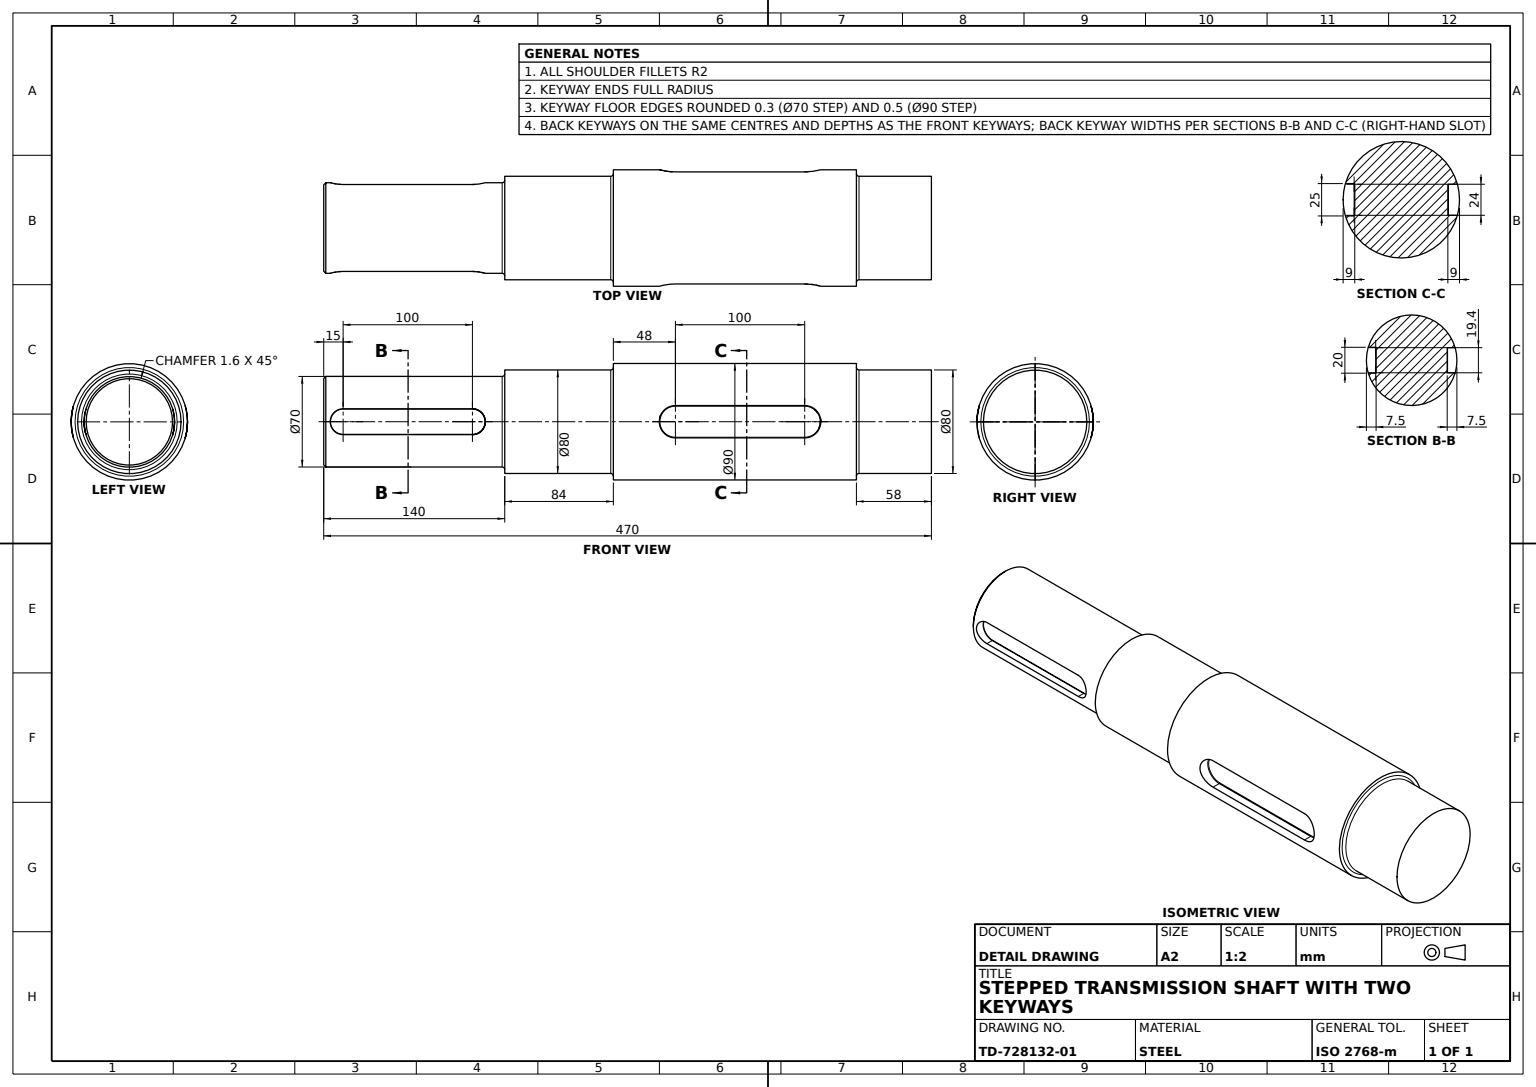
SolidWorks part; units mm, degrees
material "Plain Carbon Steel"
ref_plane "Front Plane" through (0, 0, 0) normal (0, 0, 1) x (1, 0, 0)
ref_plane "Top Plane" through (0, 0, 0) normal (0, 1, 0) x (1, 0, 0)
ref_plane "Right Plane" through (0, 0, 0) normal (1, 0, 0) x (0, 0, -1)
sketch "Shaft Profile Sketch" plane through (0, 0, 0) normal (0, 0, 1) x (1, 0, 0)
  line L0 (0, 0) -> (470, 0) construction
  line L1 (0, 0) -> (0, 35)
  line L2 (0, 35) -> (140, 35)
  line L3 (140, 35) -> (140, 40)
  line L4 (140, 40) -> (224, 40)
  line L5 (224, 40) -> (224, 45)
  line L6 (224, 45) -> (412, 45)
  line L7 (412, 45) -> (412, 40)
  line L8 (412, 40) -> (470, 40)
  line L9 (470, 40) -> (470, 0)
  line L10 (0, 0) -> (470, 0)
  dimension "D1" = 40
  dimension "D2" = 58
  dimension "D3" = 45
  dimension "D4" = 188
  dimension "D5" = 84
  dimension "D6" = 40
  dimension "D7" = 140
  dimension "D8" = 35
revolve "Stepped Shaft Body" add sketch "Shaft Profile Sketch" angle 360 about L0
chamfer "End Chamfer 1.6x45deg" distance 1.6 angle 45 1 edges at (0, 0, 35)
ref_plane "Keyway A Plane" through (0, 0, 35) normal (0, 0, 1) x (1, 0, 0)
sketch "Keyway A Sketch" plane through (0, 0, 35) normal (0, 0, 1) x (1, 0, 0)
  line L0 (15, 0) -> (115, 0) construction
  line L1 (15, 10) -> (115, 10)
  line L2 (15, -10) -> (115, -10)
  line L3 (0, 33.4) -> (0, -33.4) construction
  arc A0 (15, 10) -> (15, -10) centre (15, 0) ccw
  arc A1 (115, -10) -> (115, 10) centre (115, 0) ccw
  point P3 (65, 0)
  dimension "D2" = 10
  dimension "D1" = 100
  dimension "D3" = 15
extrude "Keyway A Cut 7.5 Deep" cut sketch "Keyway A Sketch" against normal blind 7.5
fillet "Keyway A Edge Fillet R0.3" radius 0.3 4 edges at (125, 0, 27.5) (65, -10, 27.5) (5, 0, 27.5) (65, 10, 27.5)
ref_plane "Keyway B Plane" through (0, 0, 45) normal (0, 0, 1) x (1, 0, 0)
sketch "Keyway B Sketch" plane through (0, 0, 45) normal (0, 0, 1) x (1, 0, 0)
  line L0 (272, 0) -> (372, 0) construction
  line L1 (272, 12.5) -> (372, 12.5)
  line L2 (272, -12.5) -> (372, -12.5)
  line L3 (412, -40) -> (412, 40) construction
  arc A0 (272, 12.5) -> (272, -12.5) centre (272, 0) ccw
  arc A1 (372, -12.5) -> (372, 12.5) centre (372, 0) ccw
  point P3 (322, 0)
  dimension "D2" = 12.5
  dimension "D1" = 100
  dimension "D3" = 40
extrude "Keyway B Cut 9 Deep" cut sketch "Keyway B Sketch" against normal blind 9
fillet "Keyway B Edge Fillet R0.5" radius 0.5 4 edges at (322, -12.5, 36) (259.5, 0, 36) (322, 12.5, 36) (384.5, 0, 36)
ref_plane "Keyway B Second Cut Plane" through (0, 0, -45) normal (0, 0, 1) x (1, 0, 0)
sketch "Keyway B Second Cut Sketch" plane through (0, 0, -45) normal (0, 0, 1) x (1, 0, 0)
  line L0 (372, 12) -> (272, 12) construction
  line L1 (272, -12) -> (372, -12) construction
  line L2 (372, 12) -> (272, 12)
  line L3 (272, -12) -> (372, -12)
  arc A0 (372, -12) -> (372, 12) centre (372, 0) ccw construction
  arc A1 (272, 12) -> (272, -12) centre (272, 0) ccw construction
  arc A2 (372, -12) -> (372, 12) centre (372, 0) ccw
  arc A3 (272, 12) -> (272, -12) centre (272, 0) ccw
extrude "Keyway B Second Cut" cut sketch "Keyway B Second Cut Sketch" along normal blind 9
ref_plane "Keyway A Second Cut Plane" through (0, 0, -35) normal (0, 0, 1) x (1, 0, 0)
sketch "Keyway A Second Cut Sketch" plane through (0, 0, -35) normal (0, 0, 1) x (1, 0, 0)
  line L0 (115, 9.7) -> (15, 9.7) construction
  line L1 (15, -9.7) -> (115, -9.7) construction
  line L2 (115, 9.7) -> (15, 9.7)
  line L3 (15, -9.7) -> (115, -9.7)
  arc A0 (115, -9.7) -> (115, 9.7) centre (115, 0) ccw construction
  arc A1 (15, 9.7) -> (15, -9.7) centre (15, 0) ccw construction
  arc A2 (115, -9.7) -> (115, 9.7) centre (115, 0) ccw
  arc A3 (15, 9.7) -> (15, -9.7) centre (15, 0) ccw
extrude "Keyway A Second Cut" cut sketch "Keyway A Second Cut Sketch" along normal blind 7.5
fillet "Keyway B Second Cut Fillet R0.5" radius 0.5 4 edges at (322, -12, -36) (260, 0, -36) (322, 12, -36) (384, 0, -36)
fillet "Keyway A Second Cut Fillet R0.3" radius 0.3 4 edges at (65, -9.7, -27.5) (5.3, 0, -27.5) (65, 9.7, -27.5) (124.7, 0, -27.5)
fillet "Shoulder Fillet R2" radius 2 3 edges at (412, 0, 40) (224, 0, 40) (140, 0, 35)
